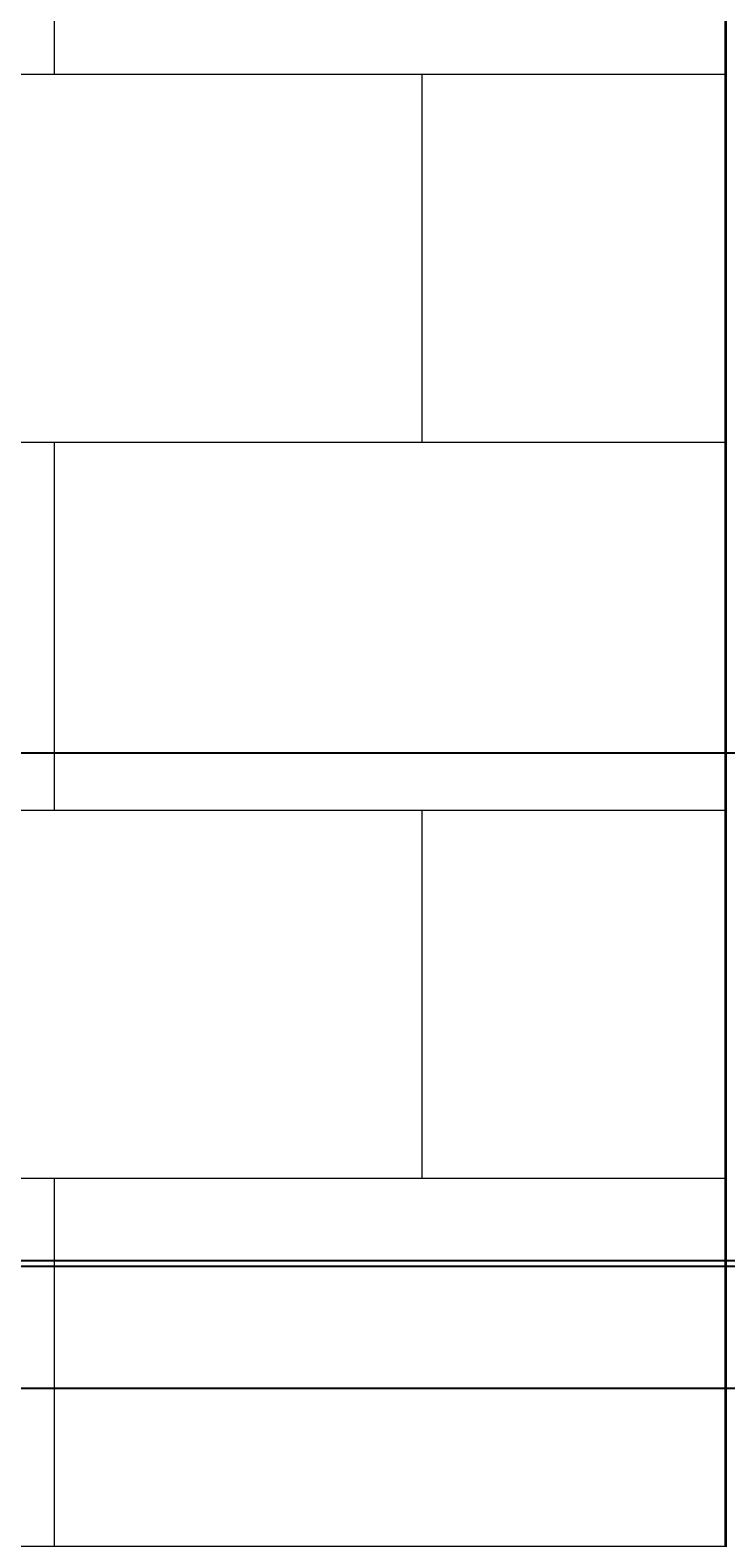
# Model space of a CAD drawing. Units: inches. Extents: x -26 to 776, y -22 to 650.
# Tile 22 of 62: x 358 to 426, y 145 to 292. Entities that reach past the tile are written whole.
import ezdxf

# ---------------------------------------------------------------- set-up
doc = ezdxf.new("R2010")
doc.units = ezdxf.units.IN
doc.header["$MEASUREMENT"] = 0
for name, color, linetype, lineweight in [('A-ANNO-DIMS', 2, 'Continuous', 18), ('A-WALL', 7, 'Continuous', 35), ('A-WALL-PATT', 8, 'Continuous', 13)]:
    doc.layers.add(name, color=color, linetype=linetype, lineweight=lineweight)
doc.styles.get("Standard").update_dxf_attribs({"font": 'arial.ttf'})
doc.dimstyles.get("Standard").update_dxf_attribs({"dimtxt": 0.5625, "dimasz": 0.18, "dimexe": 0.18, "dimexo": 0.0625, "dimgap": 0.09, "dimtad": 0, "dimtih": 1, "dimtoh": 1, "dimdec": 4, "dimzin": 0, "dimdsep": 46, "dimlunit": 4, "dimtxsty": 'Standard', "dimcen": 0.09, "dimadec": 0, "dimazin": 0, "dimtfac": 1, "dimtdec": 4, "dimtofl": 0, "dimtmove": 0, "dimatfit": 3, "dimfxl": 1, "dimtolj": 1, "dimtzin": 0, "dimarcsym": 0})

# ---------------------------------------------------------------- blocks, each defined once
blk = doc.blocks.new('*D26')
at = {"layer": 'A-ANNO-DIMS', "color": 0, "lineweight": -2, "transparency": 16777216}
for p, q in [((91.71, 171.97), (775.34, 171.97)), ((775.16, 171.79), (775.16, 166.11)), ((775.16, 159.66), (775.16, 165.35)), ((82.2, 159.48), (775.34, 159.48))]:
    blk.add_line(p, q, dxfattribs=at)
at = {"layer": 'A-ANNO-DIMS', "color": 0, "transparency": 16777216}
for points in [[(775.13, 171.79), (775.19, 171.79), (775.16, 171.97)], [(775.13, 159.66), (775.19, 159.66), (775.16, 159.48)]]:
    blk.add_solid(points, dxfattribs=at)
at = {"layer": 'Defpoints', "color": 0, "transparency": 16777216}
for p in [(91.64, 171.97), (775.16, 171.97), (82.13, 159.48)]:
    blk.add_point(p, dxfattribs=at)
at = {"layer": 'A-ANNO-DIMS', "color": 0, "transparency": 16777216, "insert": (775.16, 165.73), "char_height": 0.562, "attachment_point": 5}
blk.add_mtext('\\A1;12.49', dxfattribs=at)
blk = doc.blocks.new('*D28')
at = {"layer": 'A-ANNO-DIMS', "color": 0, "lineweight": -2, "transparency": 16777216}
for p, q in [((285.08, 314.12), (775.34, 314.12)), ((775.16, 313.94), (775.16, 243.14)), ((775.16, 171.6), (775.16, 242.4)), ((285.08, 171.42), (775.34, 171.42))]:
    blk.add_line(p, q, dxfattribs=at)
at = {"layer": 'A-ANNO-DIMS', "color": 0, "transparency": 16777216}
for points in [[(775.13, 313.94), (775.19, 313.94), (775.16, 314.12)], [(775.13, 171.6), (775.19, 171.6), (775.16, 171.42)]]:
    blk.add_solid(points, dxfattribs=at)
at = {"layer": 'Defpoints', "color": 0, "transparency": 16777216}
for p in [(285.02, 314.12), (775.16, 314.12), (285.02, 171.42)]:
    blk.add_point(p, dxfattribs=at)
at = {"layer": 'A-ANNO-DIMS', "color": 0, "transparency": 16777216, "insert": (775.16, 242.77), "char_height": 0.562, "attachment_point": 5}
blk.add_mtext('\\A1;142.7', dxfattribs=at)
blk = doc.blocks.new('*D39')
at = {"layer": 'A-ANNO-DIMS', "color": 0, "lineweight": -2, "transparency": 16777216}
for p, q in [((289.24, 15.54), (289.24, 649.86)), ((289.42, 649.68), (356.48, 649.68)), ((425.56, 649.68), (358.51, 649.68)), ((425.74, 15.54), (425.74, 649.86))]:
    blk.add_line(p, q, dxfattribs=at)
at = {"layer": 'A-ANNO-DIMS', "color": 0, "transparency": 16777216}
for points in [[(289.42, 649.71), (289.42, 649.65), (289.24, 649.68)], [(425.56, 649.71), (425.56, 649.65), (425.74, 649.68)]]:
    blk.add_solid(points, dxfattribs=at)
at = {"layer": 'Defpoints', "color": 0, "transparency": 16777216}
for p in [(425.74, 649.68), (289.24, 15.48), (425.74, 15.48)]:
    blk.add_point(p, dxfattribs=at)
at = {"layer": 'A-ANNO-DIMS', "color": 0, "transparency": 16777216, "insert": (357.49, 649.68), "char_height": 0.562, "attachment_point": 5}
blk.add_mtext('\\A1;136.5', dxfattribs=at)
blk = doc.blocks.new('*D41')
at = {"layer": 'A-ANNO-DIMS', "color": 0, "lineweight": -2, "transparency": 16777216}
for p, q in [((11.17, 221.64), (775.34, 221.64)), ((775.16, 221.46), (775.16, 190.94)), ((775.16, 159.66), (775.16, 190.18)), ((11.17, 159.48), (775.34, 159.48))]:
    blk.add_line(p, q, dxfattribs=at)
at = {"layer": 'A-ANNO-DIMS', "color": 0, "transparency": 16777216}
for points in [[(775.13, 221.46), (775.19, 221.46), (775.16, 221.64)], [(775.13, 159.66), (775.19, 159.66), (775.16, 159.48)]]:
    blk.add_solid(points, dxfattribs=at)
at = {"layer": 'Defpoints', "color": 0, "transparency": 16777216}
for p in [(11.11, 221.64), (775.16, 221.64), (11.11, 159.48)]:
    blk.add_point(p, dxfattribs=at)
at = {"layer": 'A-ANNO-DIMS', "color": 0, "transparency": 16777216, "insert": (775.16, 190.56), "char_height": 0.562, "attachment_point": 5}
blk.add_mtext('\\A1;62.16', dxfattribs=at)
blk = doc.blocks.new('*D42')
at = {"layer": 'A-ANNO-DIMS', "color": 0, "lineweight": -2, "transparency": 16777216}
for p, q in [((285.08, 171.42), (775.34, 171.42)), ((775.16, 171.24), (775.16, 165.83)), ((775.16, 159.66), (775.16, 165.07)), ((289.3, 159.48), (775.34, 159.48))]:
    blk.add_line(p, q, dxfattribs=at)
at = {"layer": 'A-ANNO-DIMS', "color": 0, "transparency": 16777216}
for points in [[(775.13, 171.24), (775.19, 171.24), (775.16, 171.42)], [(775.13, 159.66), (775.19, 159.66), (775.16, 159.48)]]:
    blk.add_solid(points, dxfattribs=at)
at = {"layer": 'Defpoints', "color": 0, "transparency": 16777216}
for p in [(285.02, 171.42), (775.16, 171.42), (289.24, 159.48)]:
    blk.add_point(p, dxfattribs=at)
at = {"layer": 'A-ANNO-DIMS', "color": 0, "transparency": 16777216, "insert": (775.16, 165.45), "char_height": 0.562, "attachment_point": 5}
blk.add_mtext('\\A1;11.935', dxfattribs=at)

msp = doc.modelspace()

# ---------------------------------------------------------------- hatches: boundary and pattern name
at = {"layer": 'A-WALL-PATT'}
h = msp.add_hatch(dxfattribs=at)
h.set_pattern_fill('AR-B816', color=256, scale=4.5)
h.paths.add_polyline_path([(425.7434, 448.2114), (289.2424, 496.9554), (289.2424, 458.1203), (289.2424, 291.1798), (289.2424, 20.7937), (425.7434, 20.7937), (425.7434, 283.2492)])

# ---------------------------------------------------------------- linework, layer by layer
at = {"layer": 'A-WALL'}
for p, q in [((425.7434, 283.2492), (425.7434, 455.4717)), ((425.7434, 15.4824), (425.7434, 283.2492))]:
    msp.add_line(p, q, dxfattribs=at)

# ---------------------------------------------------------------- dimensions: what is measured, and where the dimension line sits
at = {"layer": 'A-ANNO-DIMS'}
dim = msp.add_linear_dim(base=(425.7434, 649.6763), p1=(289.2424, 15.4824), p2=(425.7434, 15.4824), dimstyle='Standard', override={"dimdec": 1, "dimlfac": 1, "dimrnd": 0, "dimzin": 0, "dimdsep": 46, "dimlunit": 2}, dxfattribs=at)
dim.commit()
dim.dimension.update_dxf_attribs({"geometry": '*D39', "text_midpoint": (357.4929, 649.6763)})
for base, p1, p2, override, picture, middle in [((775.1553, 314.119), (285.0179, 171.4173), (285.0179, 314.119), {"dimdec": 1, "dimlfac": 1, "dimrnd": 0, "dimzin": 0, "dimdsep": 46, "dimlunit": 2}, '*D28', (775.1553, 242.7682)), ((775.1553, 221.6413), (11.1074, 159.4824), (11.1074, 221.6413), {"dimdec": 2, "dimlfac": 1, "dimrnd": 0, "dimzin": 0, "dimdsep": 46, "dimlunit": 2}, '*D41', (775.1553, 190.5618)), ((775.1553, 171.9734), (82.134, 159.4824), (91.6448, 171.9734), {"dimdec": 2, "dimlfac": 1, "dimrnd": 0, "dimzin": 0, "dimdsep": 46, "dimlunit": 2}, '*D26', (775.1553, 165.7279)), ((775.1553, 171.4173), (289.2424, 159.4824), (285.0179, 171.4173), {"dimdec": 3, "dimlfac": 1, "dimrnd": 0, "dimzin": 0, "dimdsep": 46, "dimlunit": 2}, '*D42', (775.1553, 165.4498))]:
    dim = msp.add_linear_dim(base=base, p1=p1, p2=p2, angle=90, dimstyle='Standard', override=override, dxfattribs=at)
    dim.commit()
    dim.dimension.update_dxf_attribs({"geometry": picture, "text_midpoint": middle})

doc.saveas('drawing.dxf')
